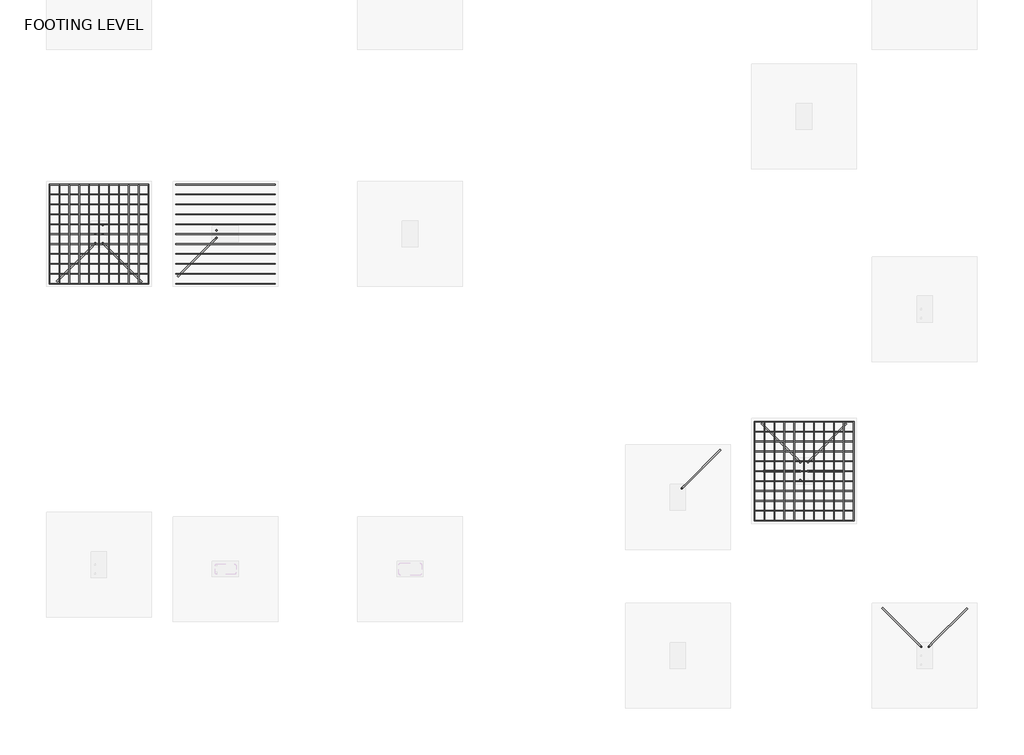
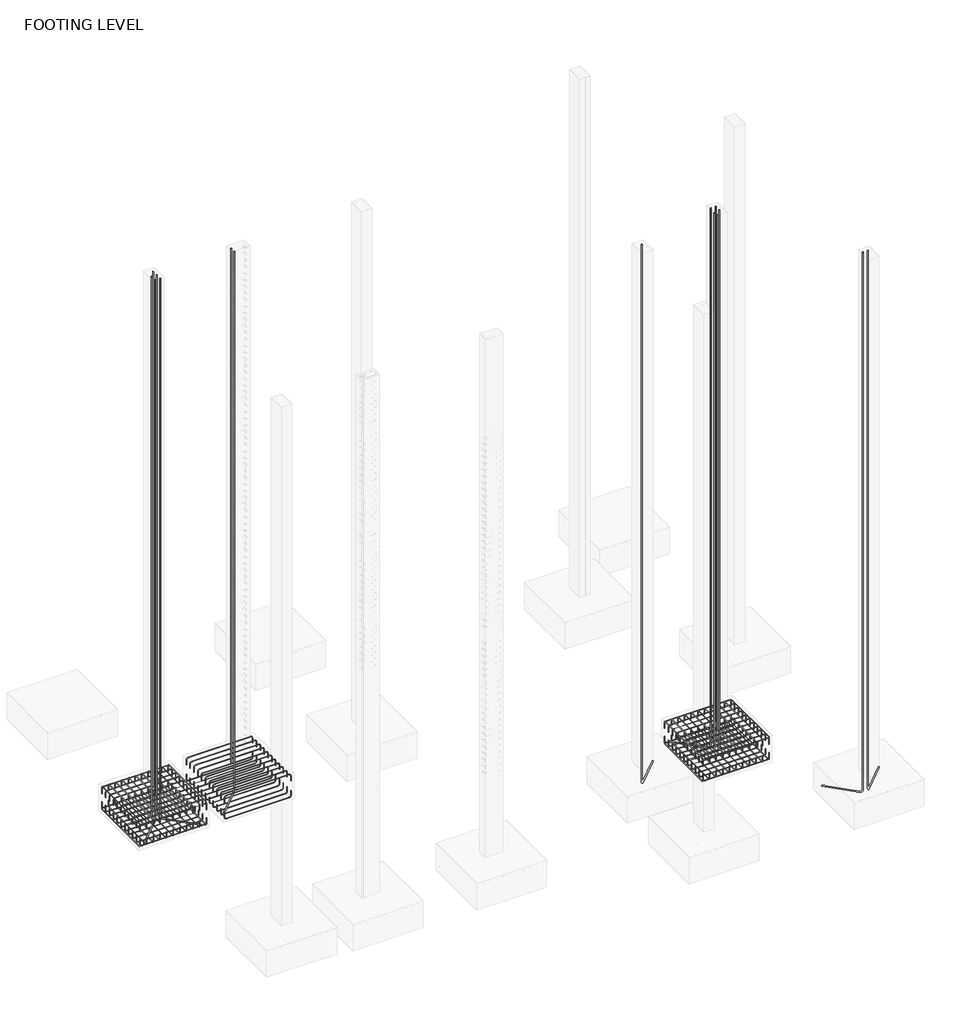
# One storey, part 7 of 10: 29 reinforcing bars.
"""IFC4 building model written with IfcOpenShell, lengths in millimetres."""

from ifc_helpers import new_model, si_unit, point, frame, origin, place, context, project, spatial, polyline, circle_curve, trimmed, segment, composite_curve, source, transform, mapped, element, save
from ifc_brep_helpers import swept_disk

model = new_model("IFC4")

# Units and contexts
model_context = context("Model", 3, world=origin())
ifc_project = project(units=[si_unit("LENGTHUNIT", "METRE", prefix="MILLI")], contexts=[model_context])

# Site, building, storey
site = spatial("IfcSite", under=ifc_project)
building = spatial("IfcBuilding", under=site)
storey = spatial("IfcBuildingStorey", under=building, Name="FOOTING LEVEL", Elevation=-1371.6)

# Reinforcing bars
placement = place(None, origin())
reinforcing_bar_shape = source(origin(), model_context, "Body", "SolidModel", [
    swept_disk(composite_curve([segment(polyline([(-13596.5793223, 10511.7953802, -1562.1), (-13596.5793223, 10511.7953802, -1447.8)]), True, "CONTINUOUS"), segment(trimmed(circle_curve(frame((-13563.2418223, 10511.7953802, -1447.8), z_axis=(0.0, 1.0, 0.0), x_axis=(-33.337499999999636, 0.0, 0.0)), 33.3375), [point((-13596.5793223, 10511.7953802, -1447.8))], [point((-13563.2418223, 10511.7953802, -1414.4625))], True, "CARTESIAN"), True, "CONTINUOUS"), segment(polyline([(-13563.2418223, 10511.7953802, -1414.4625), (-12191.6418223, 10511.7953802, -1414.4625)]), True, "CONTINUOUS"), segment(trimmed(circle_curve(frame((-12191.6418223, 10511.7953802, -1447.8), z_axis=(0.0, 1.0, 0.0), x_axis=(0.0, 0.0, 33.337499999999864)), 33.3375), [point((-12191.6418223, 10511.7953802, -1414.4625))], [point((-12158.3043223, 10511.7953802, -1447.8))], True, "CARTESIAN"), True, "CONTINUOUS"), segment(polyline([(-12158.3043223, 10511.7953802, -1447.8), (-12158.3043223, 10511.7953802, -1562.1)]), True, "CONTINUOUS")], self_intersect=False), 4.7625),
])
element("IfcReinforcingBar", 1, at=placement, inside=storey, context=model_context, shape_type="MappedRepresentation", body=[
    mapped(reinforcing_bar_shape, transform((0.0, 0.0, 0.0), x_axis=(1.0, 0.0, 0.0), y_axis=(0.0, 1.0, 0.0), z_axis=(0.0, 0.0, 1.0))),
    mapped(reinforcing_bar_shape, transform((0.0, -143.8275, 0.0), x_axis=(1.0, 0.0, 0.0), y_axis=(0.0, 1.0, 0.0), z_axis=(0.0, 0.0, 1.0))),
    mapped(reinforcing_bar_shape, transform((0.0, -287.655, 0.0), x_axis=(1.0, 0.0, 0.0), y_axis=(0.0, 1.0, 0.0), z_axis=(0.0, 0.0, 1.0))),
    mapped(reinforcing_bar_shape, transform((0.0, -431.4825, 0.0), x_axis=(1.0, 0.0, 0.0), y_axis=(0.0, 1.0, 0.0), z_axis=(0.0, 0.0, 1.0))),
    mapped(reinforcing_bar_shape, transform((0.0, -575.31, 0.0), x_axis=(1.0, 0.0, 0.0), y_axis=(0.0, 1.0, 0.0), z_axis=(0.0, 0.0, 1.0))),
    mapped(reinforcing_bar_shape, transform((0.0, -719.1375, 0.0), x_axis=(1.0, 0.0, 0.0), y_axis=(0.0, 1.0, 0.0), z_axis=(0.0, 0.0, 1.0))),
    mapped(reinforcing_bar_shape, transform((0.0, -862.965, 0.0), x_axis=(1.0, 0.0, 0.0), y_axis=(0.0, 1.0, 0.0), z_axis=(0.0, 0.0, 1.0))),
    mapped(reinforcing_bar_shape, transform((0.0, -1006.7925, 0.0), x_axis=(1.0, 0.0, 0.0), y_axis=(0.0, 1.0, 0.0), z_axis=(0.0, 0.0, 1.0))),
    mapped(reinforcing_bar_shape, transform((0.0, -1150.62, 0.0), x_axis=(1.0, 0.0, 0.0), y_axis=(0.0, 1.0, 0.0), z_axis=(0.0, 0.0, 1.0))),
    mapped(reinforcing_bar_shape, transform((0.0, -1294.4475, 0.0), x_axis=(1.0, 0.0, 0.0), y_axis=(0.0, 1.0, 0.0), z_axis=(0.0, 0.0, 1.0))),
    mapped(reinforcing_bar_shape, transform((0.0, -1438.275, 0.0), x_axis=(1.0, 0.0, 0.0), y_axis=(0.0, 1.0, 0.0), z_axis=(0.0, 0.0, 1.0))),
])
reinforcing_bar_2_shape = source(origin(), model_context, "Body", "SolidModel", [
    swept_disk(composite_curve([segment(polyline([(-12158.3043223, 10511.7953802, -1790.7), (-12158.3043223, 10511.7953802, -1905.0)]), True, "CONTINUOUS"), segment(trimmed(circle_curve(frame((-12191.6418223, 10511.7953802, -1905.0), z_axis=(0.0, 1.0, 0.0), x_axis=(33.337499999999636, 0.0, 0.0)), 33.3375), [point((-12158.3043223, 10511.7953802, -1905.0))], [point((-12191.6418223, 10511.7953802, -1938.3375))], True, "CARTESIAN"), True, "CONTINUOUS"), segment(polyline([(-12191.6418223, 10511.7953802, -1938.3375), (-13563.2418223, 10511.7953802, -1938.3375)]), True, "CONTINUOUS"), segment(trimmed(circle_curve(frame((-13563.2418223, 10511.7953802, -1905.0), z_axis=(0.0, 1.0, 0.0), x_axis=(0.0, 0.0, -33.33750000000009)), 33.3375), [point((-13563.2418223, 10511.7953802, -1938.3375))], [point((-13596.5793223, 10511.7953802, -1905.0))], True, "CARTESIAN"), True, "CONTINUOUS"), segment(polyline([(-13596.5793223, 10511.7953802, -1905.0), (-13596.5793223, 10511.7953802, -1790.7)]), True, "CONTINUOUS")], self_intersect=False), 4.7625),
])
element("IfcReinforcingBar", 2, at=placement, inside=storey, context=model_context, shape_type="MappedRepresentation", body=[
    mapped(reinforcing_bar_2_shape, transform((0.0, 0.0, 0.0), x_axis=(1.0, 0.0, 0.0), y_axis=(0.0, 1.0, 0.0), z_axis=(0.0, 0.0, 1.0))),
    mapped(reinforcing_bar_2_shape, transform((0.0, -143.8275, 0.0), x_axis=(1.0, 0.0, 0.0), y_axis=(0.0, 1.0, 0.0), z_axis=(0.0, 0.0, 1.0))),
    mapped(reinforcing_bar_2_shape, transform((0.0, -287.655, 0.0), x_axis=(1.0, 0.0, 0.0), y_axis=(0.0, 1.0, 0.0), z_axis=(0.0, 0.0, 1.0))),
    mapped(reinforcing_bar_2_shape, transform((0.0, -431.4825, 0.0), x_axis=(1.0, 0.0, 0.0), y_axis=(0.0, 1.0, 0.0), z_axis=(0.0, 0.0, 1.0))),
    mapped(reinforcing_bar_2_shape, transform((0.0, -575.31, 0.0), x_axis=(1.0, 0.0, 0.0), y_axis=(0.0, 1.0, 0.0), z_axis=(0.0, 0.0, 1.0))),
    mapped(reinforcing_bar_2_shape, transform((0.0, -719.1375, 0.0), x_axis=(1.0, 0.0, 0.0), y_axis=(0.0, 1.0, 0.0), z_axis=(0.0, 0.0, 1.0))),
    mapped(reinforcing_bar_2_shape, transform((0.0, -862.965, 0.0), x_axis=(1.0, 0.0, 0.0), y_axis=(0.0, 1.0, 0.0), z_axis=(0.0, 0.0, 1.0))),
    mapped(reinforcing_bar_2_shape, transform((0.0, -1006.7925, 0.0), x_axis=(1.0, 0.0, 0.0), y_axis=(0.0, 1.0, 0.0), z_axis=(0.0, 0.0, 1.0))),
    mapped(reinforcing_bar_2_shape, transform((0.0, -1150.62, 0.0), x_axis=(1.0, 0.0, 0.0), y_axis=(0.0, 1.0, 0.0), z_axis=(0.0, 0.0, 1.0))),
    mapped(reinforcing_bar_2_shape, transform((0.0, -1294.4475, 0.0), x_axis=(1.0, 0.0, 0.0), y_axis=(0.0, 1.0, 0.0), z_axis=(0.0, 0.0, 1.0))),
    mapped(reinforcing_bar_2_shape, transform((0.0, -1438.275, 0.0), x_axis=(1.0, 0.0, 0.0), y_axis=(0.0, 1.0, 0.0), z_axis=(0.0, 0.0, 1.0))),
])
reinforcing_bar_3_shape = source(origin(), model_context, "Body", "SolidModel", [
    swept_disk(composite_curve([segment(polyline([(-13993.4543223, 10511.7953802, -1562.1), (-13993.4543223, 10511.7953802, -1447.8)]), True, "CONTINUOUS"), segment(trimmed(circle_curve(frame((-13993.4543223, 10478.4578802, -1447.8), z_axis=(1.0, 0.0, 0.0), x_axis=(0.0, 33.337499999999636, 0.0)), 33.3375), [point((-13993.4543223, 10511.7953802, -1447.8))], [point((-13993.4543223, 10478.4578802, -1414.4625))], True, "CARTESIAN"), True, "CONTINUOUS"), segment(polyline([(-13993.4543223, 10478.4578802, -1414.4625), (-13993.4543223, 9106.8578802, -1414.4625)]), True, "CONTINUOUS"), segment(trimmed(circle_curve(frame((-13993.4543223, 9106.8578802, -1447.8), z_axis=(1.0, 0.0, 0.0), x_axis=(0.0, 0.0, 33.337499999999864)), 33.3375), [point((-13993.4543223, 9106.8578802, -1414.4625))], [point((-13993.4543223, 9073.5203802, -1447.8))], True, "CARTESIAN"), True, "CONTINUOUS"), segment(polyline([(-13993.4543223, 9073.5203802, -1447.8), (-13993.4543223, 9073.5203802, -1562.1)]), True, "CONTINUOUS")], self_intersect=False), 4.7625),
])
element("IfcReinforcingBar", 3, at=placement, inside=storey, context=model_context, shape_type="MappedRepresentation", body=[
    mapped(reinforcing_bar_3_shape, transform((0.0, 0.0, 0.0), x_axis=(1.0, 0.0, 0.0), y_axis=(0.0, 1.0, 0.0), z_axis=(0.0, 0.0, 1.0))),
    mapped(reinforcing_bar_3_shape, transform((-143.8275, 0.0, 0.0), x_axis=(1.0, 0.0, 0.0), y_axis=(0.0, 1.0, 0.0), z_axis=(0.0, 0.0, 1.0))),
    mapped(reinforcing_bar_3_shape, transform((-287.655, 0.0, 0.0), x_axis=(1.0, 0.0, 0.0), y_axis=(0.0, 1.0, 0.0), z_axis=(0.0, 0.0, 1.0))),
    mapped(reinforcing_bar_3_shape, transform((-431.4825, 0.0, 0.0), x_axis=(1.0, 0.0, 0.0), y_axis=(0.0, 1.0, 0.0), z_axis=(0.0, 0.0, 1.0))),
    mapped(reinforcing_bar_3_shape, transform((-575.31, 0.0, 0.0), x_axis=(1.0, 0.0, 0.0), y_axis=(0.0, 1.0, 0.0), z_axis=(0.0, 0.0, 1.0))),
    mapped(reinforcing_bar_3_shape, transform((-719.1375, 0.0, 0.0), x_axis=(1.0, 0.0, 0.0), y_axis=(0.0, 1.0, 0.0), z_axis=(0.0, 0.0, 1.0))),
    mapped(reinforcing_bar_3_shape, transform((-862.965, 0.0, 0.0), x_axis=(1.0, 0.0, 0.0), y_axis=(0.0, 1.0, 0.0), z_axis=(0.0, 0.0, 1.0))),
    mapped(reinforcing_bar_3_shape, transform((-1006.7925, 0.0, 0.0), x_axis=(1.0, 0.0, 0.0), y_axis=(0.0, 1.0, 0.0), z_axis=(0.0, 0.0, 1.0))),
    mapped(reinforcing_bar_3_shape, transform((-1150.62, 0.0, 0.0), x_axis=(1.0, 0.0, 0.0), y_axis=(0.0, 1.0, 0.0), z_axis=(0.0, 0.0, 1.0))),
    mapped(reinforcing_bar_3_shape, transform((-1294.4475, 0.0, 0.0), x_axis=(1.0, 0.0, 0.0), y_axis=(0.0, 1.0, 0.0), z_axis=(0.0, 0.0, 1.0))),
    mapped(reinforcing_bar_3_shape, transform((-1438.275, 0.0, 0.0), x_axis=(1.0, 0.0, 0.0), y_axis=(0.0, 1.0, 0.0), z_axis=(0.0, 0.0, 1.0))),
])
reinforcing_bar_4_shape = source(origin(), model_context, "Body", "SolidModel", [
    swept_disk(composite_curve([segment(polyline([(-13993.4543223, 9073.5203802, -1790.7), (-13993.4543223, 9073.5203802, -1905.0)]), True, "CONTINUOUS"), segment(trimmed(circle_curve(frame((-13993.4543223, 9106.8578802, -1905.0), z_axis=(1.0, 0.0, 0.0), x_axis=(0.0, -33.337499999999636, 0.0)), 33.3375), [point((-13993.4543223, 9073.5203802, -1905.0))], [point((-13993.4543223, 9106.8578802, -1938.3375))], True, "CARTESIAN"), True, "CONTINUOUS"), segment(polyline([(-13993.4543223, 9106.8578802, -1938.3375), (-13993.4543223, 10478.4578802, -1938.3375)]), True, "CONTINUOUS"), segment(trimmed(circle_curve(frame((-13993.4543223, 10478.4578802, -1905.0), z_axis=(1.0, 0.0, 0.0), x_axis=(0.0, 0.0, -33.33750000000009)), 33.3375), [point((-13993.4543223, 10478.4578802, -1938.3375))], [point((-13993.4543223, 10511.7953802, -1905.0))], True, "CARTESIAN"), True, "CONTINUOUS"), segment(polyline([(-13993.4543223, 10511.7953802, -1905.0), (-13993.4543223, 10511.7953802, -1790.7)]), True, "CONTINUOUS")], self_intersect=False), 4.7625),
])
element("IfcReinforcingBar", 4, at=placement, inside=storey, context=model_context, shape_type="MappedRepresentation", body=[
    mapped(reinforcing_bar_4_shape, transform((0.0, 0.0, 0.0), x_axis=(1.0, 0.0, 0.0), y_axis=(0.0, 1.0, 0.0), z_axis=(0.0, 0.0, 1.0))),
    mapped(reinforcing_bar_4_shape, transform((-143.8275, 0.0, 0.0), x_axis=(1.0, 0.0, 0.0), y_axis=(0.0, 1.0, 0.0), z_axis=(0.0, 0.0, 1.0))),
    mapped(reinforcing_bar_4_shape, transform((-287.655, 0.0, 0.0), x_axis=(1.0, 0.0, 0.0), y_axis=(0.0, 1.0, 0.0), z_axis=(0.0, 0.0, 1.0))),
    mapped(reinforcing_bar_4_shape, transform((-431.4825, 0.0, 0.0), x_axis=(1.0, 0.0, 0.0), y_axis=(0.0, 1.0, 0.0), z_axis=(0.0, 0.0, 1.0))),
    mapped(reinforcing_bar_4_shape, transform((-575.31, 0.0, 0.0), x_axis=(1.0, 0.0, 0.0), y_axis=(0.0, 1.0, 0.0), z_axis=(0.0, 0.0, 1.0))),
    mapped(reinforcing_bar_4_shape, transform((-719.1375, 0.0, 0.0), x_axis=(1.0, 0.0, 0.0), y_axis=(0.0, 1.0, 0.0), z_axis=(0.0, 0.0, 1.0))),
    mapped(reinforcing_bar_4_shape, transform((-862.965, 0.0, 0.0), x_axis=(1.0, 0.0, 0.0), y_axis=(0.0, 1.0, 0.0), z_axis=(0.0, 0.0, 1.0))),
    mapped(reinforcing_bar_4_shape, transform((-1006.7925, 0.0, 0.0), x_axis=(1.0, 0.0, 0.0), y_axis=(0.0, 1.0, 0.0), z_axis=(0.0, 0.0, 1.0))),
    mapped(reinforcing_bar_4_shape, transform((-1150.62, 0.0, 0.0), x_axis=(1.0, 0.0, 0.0), y_axis=(0.0, 1.0, 0.0), z_axis=(0.0, 0.0, 1.0))),
    mapped(reinforcing_bar_4_shape, transform((-1294.4475, 0.0, 0.0), x_axis=(1.0, 0.0, 0.0), y_axis=(0.0, 1.0, 0.0), z_axis=(0.0, 0.0, 1.0))),
    mapped(reinforcing_bar_4_shape, transform((-1438.275, 0.0, 0.0), x_axis=(1.0, 0.0, 0.0), y_axis=(0.0, 1.0, 0.0), z_axis=(0.0, 0.0, 1.0))),
])
reinforcing_bar_5_shape = source(origin(), model_context, "Body", "SolidModel", [
    swept_disk(composite_curve([segment(polyline([(-15431.7293223, 9073.5203802, -1770.864029), (-15431.7293223, 9073.5203802, -1885.164029)]), True, "CONTINUOUS"), segment(trimmed(circle_curve(frame((-15398.3918223, 9073.5203802, -1885.164029), z_axis=(0.0, -1.0, 0.0), x_axis=(-33.337499999999636, 0.0, 0.0)), 33.3375), [point((-15431.7293223, 9073.5203802, -1885.164029))], [point((-15398.3918223, 9073.5203802, -1918.501529))], True, "CARTESIAN"), True, "CONTINUOUS"), segment(polyline([(-15398.3918223, 9073.5203802, -1918.501529), (-14026.7918223, 9073.5203802, -1918.501529)]), True, "CONTINUOUS"), segment(trimmed(circle_curve(frame((-14026.7918223, 9073.5203802, -1885.164029), z_axis=(0.0, -1.0, 0.0), x_axis=(0.0, 0.0, -33.337499999999864)), 33.3375), [point((-14026.7918223, 9073.5203802, -1918.501529))], [point((-13993.4543223, 9073.5203802, -1885.164029))], True, "CARTESIAN"), True, "CONTINUOUS"), segment(polyline([(-13993.4543223, 9073.5203802, -1885.164029), (-13993.4543223, 9073.5203802, -1770.864029)]), True, "CONTINUOUS")], self_intersect=False), 4.7625),
])
element("IfcReinforcingBar", 5, at=placement, inside=storey, context=model_context, shape_type="MappedRepresentation", body=[
    mapped(reinforcing_bar_5_shape, transform((0.0, 0.0, 0.0), x_axis=(1.0, 0.0, 0.0), y_axis=(0.0, 1.0, 0.0), z_axis=(0.0, 0.0, 1.0))),
    mapped(reinforcing_bar_5_shape, transform((0.0, 143.8275, 0.0), x_axis=(1.0, 0.0, 0.0), y_axis=(0.0, 1.0, 0.0), z_axis=(0.0, 0.0, 1.0))),
    mapped(reinforcing_bar_5_shape, transform((0.0, 287.655, 0.0), x_axis=(1.0, 0.0, 0.0), y_axis=(0.0, 1.0, 0.0), z_axis=(0.0, 0.0, 1.0))),
    mapped(reinforcing_bar_5_shape, transform((0.0, 431.4825, 0.0), x_axis=(1.0, 0.0, 0.0), y_axis=(0.0, 1.0, 0.0), z_axis=(0.0, 0.0, 1.0))),
    mapped(reinforcing_bar_5_shape, transform((0.0, 575.31, 0.0), x_axis=(1.0, 0.0, 0.0), y_axis=(0.0, 1.0, 0.0), z_axis=(0.0, 0.0, 1.0))),
    mapped(reinforcing_bar_5_shape, transform((0.0, 719.1375, 0.0), x_axis=(1.0, 0.0, 0.0), y_axis=(0.0, 1.0, 0.0), z_axis=(0.0, 0.0, 1.0))),
    mapped(reinforcing_bar_5_shape, transform((0.0, 862.965, 0.0), x_axis=(1.0, 0.0, 0.0), y_axis=(0.0, 1.0, 0.0), z_axis=(0.0, 0.0, 1.0))),
    mapped(reinforcing_bar_5_shape, transform((0.0, 1006.7925, 0.0), x_axis=(1.0, 0.0, 0.0), y_axis=(0.0, 1.0, 0.0), z_axis=(0.0, 0.0, 1.0))),
    mapped(reinforcing_bar_5_shape, transform((0.0, 1150.62, 0.0), x_axis=(1.0, 0.0, 0.0), y_axis=(0.0, 1.0, 0.0), z_axis=(0.0, 0.0, 1.0))),
    mapped(reinforcing_bar_5_shape, transform((0.0, 1294.4475, 0.0), x_axis=(1.0, 0.0, 0.0), y_axis=(0.0, 1.0, 0.0), z_axis=(0.0, 0.0, 1.0))),
    mapped(reinforcing_bar_5_shape, transform((0.0, 1438.275, 0.0), x_axis=(1.0, 0.0, 0.0), y_axis=(0.0, 1.0, 0.0), z_axis=(0.0, 0.0, 1.0))),
])
reinforcing_bar_6_shape = source(origin(), model_context, "Body", "SolidModel", [
    swept_disk(composite_curve([segment(polyline([(-15431.7293223, 10511.7953802, -1586.5406765), (-15431.7293223, 10511.7953802, -1472.2406765)]), True, "CONTINUOUS"), segment(trimmed(circle_curve(frame((-15398.3918223, 10511.7953802, -1472.2406765), z_axis=(0.0, 1.0, 0.0), x_axis=(-33.337499999999636, 0.0, 0.0)), 33.3375), [point((-15431.7293223, 10511.7953802, -1472.2406765))], [point((-15398.3918223, 10511.7953802, -1438.9031765))], True, "CARTESIAN"), True, "CONTINUOUS"), segment(polyline([(-15398.3918223, 10511.7953802, -1438.9031765), (-14026.7918223, 10511.7953802, -1438.9031765)]), True, "CONTINUOUS"), segment(trimmed(circle_curve(frame((-14026.7918223, 10511.7953802, -1472.2406765), z_axis=(0.0, 1.0, 0.0), x_axis=(0.0, 0.0, 33.33750000000009)), 33.3375), [point((-14026.7918223, 10511.7953802, -1438.9031765))], [point((-13993.4543223, 10511.7953802, -1472.2406765))], True, "CARTESIAN"), True, "CONTINUOUS"), segment(polyline([(-13993.4543223, 10511.7953802, -1472.2406765), (-13993.4543223, 10511.7953802, -1586.5406765)]), True, "CONTINUOUS")], self_intersect=False), 4.7625),
])
element("IfcReinforcingBar", 6, at=placement, inside=storey, context=model_context, shape_type="MappedRepresentation", body=[
    mapped(reinforcing_bar_6_shape, transform((0.0, 0.0, 0.0), x_axis=(1.0, 0.0, 0.0), y_axis=(0.0, 1.0, 0.0), z_axis=(0.0, 0.0, 1.0))),
    mapped(reinforcing_bar_6_shape, transform((0.0, -143.8275, 0.0), x_axis=(1.0, 0.0, 0.0), y_axis=(0.0, 1.0, 0.0), z_axis=(0.0, 0.0, 1.0))),
    mapped(reinforcing_bar_6_shape, transform((0.0, -287.655, 0.0), x_axis=(1.0, 0.0, 0.0), y_axis=(0.0, 1.0, 0.0), z_axis=(0.0, 0.0, 1.0))),
    mapped(reinforcing_bar_6_shape, transform((0.0, -431.4825, 0.0), x_axis=(1.0, 0.0, 0.0), y_axis=(0.0, 1.0, 0.0), z_axis=(0.0, 0.0, 1.0))),
    mapped(reinforcing_bar_6_shape, transform((0.0, -575.31, 0.0), x_axis=(1.0, 0.0, 0.0), y_axis=(0.0, 1.0, 0.0), z_axis=(0.0, 0.0, 1.0))),
    mapped(reinforcing_bar_6_shape, transform((0.0, -719.1375, 0.0), x_axis=(1.0, 0.0, 0.0), y_axis=(0.0, 1.0, 0.0), z_axis=(0.0, 0.0, 1.0))),
    mapped(reinforcing_bar_6_shape, transform((0.0, -862.965, 0.0), x_axis=(1.0, 0.0, 0.0), y_axis=(0.0, 1.0, 0.0), z_axis=(0.0, 0.0, 1.0))),
    mapped(reinforcing_bar_6_shape, transform((0.0, -1006.7925, 0.0), x_axis=(1.0, 0.0, 0.0), y_axis=(0.0, 1.0, 0.0), z_axis=(0.0, 0.0, 1.0))),
    mapped(reinforcing_bar_6_shape, transform((0.0, -1150.62, 0.0), x_axis=(1.0, 0.0, 0.0), y_axis=(0.0, 1.0, 0.0), z_axis=(0.0, 0.0, 1.0))),
    mapped(reinforcing_bar_6_shape, transform((0.0, -1294.4475, 0.0), x_axis=(1.0, 0.0, 0.0), y_axis=(0.0, 1.0, 0.0), z_axis=(0.0, 0.0, 1.0))),
    mapped(reinforcing_bar_6_shape, transform((0.0, -1438.275, 0.0), x_axis=(1.0, 0.0, 0.0), y_axis=(0.0, 1.0, 0.0), z_axis=(0.0, 0.0, 1.0))),
])
reinforcing_bar_7_shape = source(origin(), model_context, "Body", "SolidModel", [
    swept_disk(composite_curve([segment(polyline([(-5201.8793223, 5631.8203802, -1562.1), (-5201.8793223, 5631.8203802, -1447.8)]), True, "CONTINUOUS"), segment(trimmed(circle_curve(frame((-5201.8793223, 5665.1578802, -1447.8), z_axis=(-1.0, 0.0, 0.0), x_axis=(0.0, -33.337500000000546, 0.0)), 33.3375), [point((-5201.8793223, 5631.8203802, -1447.8))], [point((-5201.8793223, 5665.1578802, -1414.4625))], True, "CARTESIAN"), True, "CONTINUOUS"), segment(polyline([(-5201.8793223, 5665.1578802, -1414.4625), (-5201.8793223, 7036.7578802, -1414.4625)]), True, "CONTINUOUS"), segment(trimmed(circle_curve(frame((-5201.8793223, 7036.7578802, -1447.8), z_axis=(-1.0, 0.0, 0.0), x_axis=(0.0, 0.0, 33.337499999999864)), 33.3375), [point((-5201.8793223, 7036.7578802, -1414.4625))], [point((-5201.8793223, 7070.0953802, -1447.8))], True, "CARTESIAN"), True, "CONTINUOUS"), segment(polyline([(-5201.8793223, 7070.0953802, -1447.8), (-5201.8793223, 7070.0953802, -1562.1)]), True, "CONTINUOUS")], self_intersect=False), 4.7625),
])
element("IfcReinforcingBar", 7, at=placement, inside=storey, context=model_context, shape_type="MappedRepresentation", body=[
    mapped(reinforcing_bar_7_shape, transform((0.0, 0.0, 0.0), x_axis=(1.0, 0.0, 0.0), y_axis=(0.0, 1.0, 0.0), z_axis=(0.0, 0.0, 1.0))),
    mapped(reinforcing_bar_7_shape, transform((143.8275, 0.0, 0.0), x_axis=(1.0, 0.0, 0.0), y_axis=(0.0, 1.0, 0.0), z_axis=(0.0, 0.0, 1.0))),
    mapped(reinforcing_bar_7_shape, transform((287.655, 0.0, 0.0), x_axis=(1.0, 0.0, 0.0), y_axis=(0.0, 1.0, 0.0), z_axis=(0.0, 0.0, 1.0))),
    mapped(reinforcing_bar_7_shape, transform((431.4825, 0.0, 0.0), x_axis=(1.0, 0.0, 0.0), y_axis=(0.0, 1.0, 0.0), z_axis=(0.0, 0.0, 1.0))),
    mapped(reinforcing_bar_7_shape, transform((575.31, 0.0, 0.0), x_axis=(1.0, 0.0, 0.0), y_axis=(0.0, 1.0, 0.0), z_axis=(0.0, 0.0, 1.0))),
    mapped(reinforcing_bar_7_shape, transform((719.1375, 0.0, 0.0), x_axis=(1.0, 0.0, 0.0), y_axis=(0.0, 1.0, 0.0), z_axis=(0.0, 0.0, 1.0))),
    mapped(reinforcing_bar_7_shape, transform((862.965, 0.0, 0.0), x_axis=(1.0, 0.0, 0.0), y_axis=(0.0, 1.0, 0.0), z_axis=(0.0, 0.0, 1.0))),
    mapped(reinforcing_bar_7_shape, transform((1006.7925, 0.0, 0.0), x_axis=(1.0, 0.0, 0.0), y_axis=(0.0, 1.0, 0.0), z_axis=(0.0, 0.0, 1.0))),
    mapped(reinforcing_bar_7_shape, transform((1150.62, 0.0, 0.0), x_axis=(1.0, 0.0, 0.0), y_axis=(0.0, 1.0, 0.0), z_axis=(0.0, 0.0, 1.0))),
    mapped(reinforcing_bar_7_shape, transform((1294.4475, 0.0, 0.0), x_axis=(1.0, 0.0, 0.0), y_axis=(0.0, 1.0, 0.0), z_axis=(0.0, 0.0, 1.0))),
    mapped(reinforcing_bar_7_shape, transform((1438.275, 0.0, 0.0), x_axis=(1.0, 0.0, 0.0), y_axis=(0.0, 1.0, 0.0), z_axis=(0.0, 0.0, 1.0))),
])
reinforcing_bar_8_shape = source(origin(), model_context, "Body", "SolidModel", [
    swept_disk(composite_curve([segment(polyline([(-5201.8793223, 7070.0953802, -1790.7), (-5201.8793223, 7070.0953802, -1905.0)]), True, "CONTINUOUS"), segment(trimmed(circle_curve(frame((-5201.8793223, 7036.7578802, -1905.0), z_axis=(-1.0, 0.0, 0.0), x_axis=(0.0, 33.337500000000546, 0.0)), 33.3375), [point((-5201.8793223, 7070.0953802, -1905.0))], [point((-5201.8793223, 7036.7578802, -1938.3375))], True, "CARTESIAN"), True, "CONTINUOUS"), segment(polyline([(-5201.8793223, 7036.7578802, -1938.3375), (-5201.8793223, 5665.1578802, -1938.3375)]), True, "CONTINUOUS"), segment(trimmed(circle_curve(frame((-5201.8793223, 5665.1578802, -1905.0), z_axis=(-1.0, 0.0, 0.0), x_axis=(0.0, 0.0, -33.33750000000009)), 33.3375), [point((-5201.8793223, 5665.1578802, -1938.3375))], [point((-5201.8793223, 5631.8203802, -1905.0))], True, "CARTESIAN"), True, "CONTINUOUS"), segment(polyline([(-5201.8793223, 5631.8203802, -1905.0), (-5201.8793223, 5631.8203802, -1790.7)]), True, "CONTINUOUS")], self_intersect=False), 4.7625),
])
element("IfcReinforcingBar", 8, at=placement, inside=storey, context=model_context, shape_type="MappedRepresentation", body=[
    mapped(reinforcing_bar_8_shape, transform((0.0, 0.0, 0.0), x_axis=(1.0, 0.0, 0.0), y_axis=(0.0, 1.0, 0.0), z_axis=(0.0, 0.0, 1.0))),
    mapped(reinforcing_bar_8_shape, transform((143.8275, 0.0, 0.0), x_axis=(1.0, 0.0, 0.0), y_axis=(0.0, 1.0, 0.0), z_axis=(0.0, 0.0, 1.0))),
    mapped(reinforcing_bar_8_shape, transform((287.655, 0.0, 0.0), x_axis=(1.0, 0.0, 0.0), y_axis=(0.0, 1.0, 0.0), z_axis=(0.0, 0.0, 1.0))),
    mapped(reinforcing_bar_8_shape, transform((431.4825, 0.0, 0.0), x_axis=(1.0, 0.0, 0.0), y_axis=(0.0, 1.0, 0.0), z_axis=(0.0, 0.0, 1.0))),
    mapped(reinforcing_bar_8_shape, transform((575.31, 0.0, 0.0), x_axis=(1.0, 0.0, 0.0), y_axis=(0.0, 1.0, 0.0), z_axis=(0.0, 0.0, 1.0))),
    mapped(reinforcing_bar_8_shape, transform((719.1375, 0.0, 0.0), x_axis=(1.0, 0.0, 0.0), y_axis=(0.0, 1.0, 0.0), z_axis=(0.0, 0.0, 1.0))),
    mapped(reinforcing_bar_8_shape, transform((862.965, 0.0, 0.0), x_axis=(1.0, 0.0, 0.0), y_axis=(0.0, 1.0, 0.0), z_axis=(0.0, 0.0, 1.0))),
    mapped(reinforcing_bar_8_shape, transform((1006.7925, 0.0, 0.0), x_axis=(1.0, 0.0, 0.0), y_axis=(0.0, 1.0, 0.0), z_axis=(0.0, 0.0, 1.0))),
    mapped(reinforcing_bar_8_shape, transform((1150.62, 0.0, 0.0), x_axis=(1.0, 0.0, 0.0), y_axis=(0.0, 1.0, 0.0), z_axis=(0.0, 0.0, 1.0))),
    mapped(reinforcing_bar_8_shape, transform((1294.4475, 0.0, 0.0), x_axis=(1.0, 0.0, 0.0), y_axis=(0.0, 1.0, 0.0), z_axis=(0.0, 0.0, 1.0))),
    mapped(reinforcing_bar_8_shape, transform((1438.275, 0.0, 0.0), x_axis=(1.0, 0.0, 0.0), y_axis=(0.0, 1.0, 0.0), z_axis=(0.0, 0.0, 1.0))),
])
reinforcing_bar_9_shape = source(origin(), model_context, "Body", "SolidModel", [
    swept_disk(composite_curve([segment(polyline([(-3763.6043223, 7070.0953802, -1770.864029), (-3763.6043223, 7070.0953802, -1885.164029)]), True, "CONTINUOUS"), segment(trimmed(circle_curve(frame((-3796.9418223, 7070.0953802, -1885.164029), z_axis=(0.0, 1.0, 0.0), x_axis=(33.337499999999636, 0.0, 0.0)), 33.3375), [point((-3763.6043223, 7070.0953802, -1885.164029))], [point((-3796.9418223, 7070.0953802, -1918.501529))], True, "CARTESIAN"), True, "CONTINUOUS"), segment(polyline([(-3796.9418223, 7070.0953802, -1918.501529), (-5168.5418223, 7070.0953802, -1918.501529)]), True, "CONTINUOUS"), segment(trimmed(circle_curve(frame((-5168.5418223, 7070.0953802, -1885.164029), z_axis=(0.0, 1.0, 0.0), x_axis=(0.0, 0.0, -33.337499999999864)), 33.3375), [point((-5168.5418223, 7070.0953802, -1918.501529))], [point((-5201.8793223, 7070.0953802, -1885.164029))], True, "CARTESIAN"), True, "CONTINUOUS"), segment(polyline([(-5201.8793223, 7070.0953802, -1885.164029), (-5201.8793223, 7070.0953802, -1770.864029)]), True, "CONTINUOUS")], self_intersect=False), 4.7625),
])
element("IfcReinforcingBar", 9, at=placement, inside=storey, context=model_context, shape_type="MappedRepresentation", body=[
    mapped(reinforcing_bar_9_shape, transform((0.0, 0.0, 0.0), x_axis=(1.0, 0.0, 0.0), y_axis=(0.0, 1.0, 0.0), z_axis=(0.0, 0.0, 1.0))),
    mapped(reinforcing_bar_9_shape, transform((0.0, -143.8275, 0.0), x_axis=(1.0, 0.0, 0.0), y_axis=(0.0, 1.0, 0.0), z_axis=(0.0, 0.0, 1.0))),
    mapped(reinforcing_bar_9_shape, transform((0.0, -287.655, 0.0), x_axis=(1.0, 0.0, 0.0), y_axis=(0.0, 1.0, 0.0), z_axis=(0.0, 0.0, 1.0))),
    mapped(reinforcing_bar_9_shape, transform((0.0, -431.4825, 0.0), x_axis=(1.0, 0.0, 0.0), y_axis=(0.0, 1.0, 0.0), z_axis=(0.0, 0.0, 1.0))),
    mapped(reinforcing_bar_9_shape, transform((0.0, -575.31, 0.0), x_axis=(1.0, 0.0, 0.0), y_axis=(0.0, 1.0, 0.0), z_axis=(0.0, 0.0, 1.0))),
    mapped(reinforcing_bar_9_shape, transform((0.0, -719.1375, 0.0), x_axis=(1.0, 0.0, 0.0), y_axis=(0.0, 1.0, 0.0), z_axis=(0.0, 0.0, 1.0))),
    mapped(reinforcing_bar_9_shape, transform((0.0, -862.965, 0.0), x_axis=(1.0, 0.0, 0.0), y_axis=(0.0, 1.0, 0.0), z_axis=(0.0, 0.0, 1.0))),
    mapped(reinforcing_bar_9_shape, transform((0.0, -1006.7925, 0.0), x_axis=(1.0, 0.0, 0.0), y_axis=(0.0, 1.0, 0.0), z_axis=(0.0, 0.0, 1.0))),
    mapped(reinforcing_bar_9_shape, transform((0.0, -1150.62, 0.0), x_axis=(1.0, 0.0, 0.0), y_axis=(0.0, 1.0, 0.0), z_axis=(0.0, 0.0, 1.0))),
    mapped(reinforcing_bar_9_shape, transform((0.0, -1294.4475, 0.0), x_axis=(1.0, 0.0, 0.0), y_axis=(0.0, 1.0, 0.0), z_axis=(0.0, 0.0, 1.0))),
    mapped(reinforcing_bar_9_shape, transform((0.0, -1438.275, 0.0), x_axis=(1.0, 0.0, 0.0), y_axis=(0.0, 1.0, 0.0), z_axis=(0.0, 0.0, 1.0))),
])
element("IfcReinforcingBar", 10, at=placement, inside=storey, context=model_context, shape_type="SolidModel", body=[
    swept_disk(composite_curve([segment(polyline([(-14658.2316302, 9923.2180723, -1333.5), (-14658.2316302, 9923.2180723, 10477.5)]), True, "CONTINUOUS")], self_intersect=False), 9.525),
])
element("IfcReinforcingBar", 11, at=placement, inside=storey, context=model_context, shape_type="SolidModel", body=[
    swept_disk(composite_curve([segment(polyline([(-14766.9520144, 9662.0976881, -1333.5), (-14766.9520144, 9662.0976881, 10477.5)]), True, "CONTINUOUS")], self_intersect=False), 9.525),
])
element("IfcReinforcingBar", 12, at=placement, inside=storey, context=model_context, shape_type="SolidModel", body=[
    swept_disk(composite_curve([segment(polyline([(-14658.2316302, 9662.0976881, -1333.5), (-14658.2316302, 9662.0976881, 10477.5)]), True, "CONTINUOUS")], self_intersect=False), 9.525),
])
element("IfcReinforcingBar", 13, at=placement, inside=storey, context=model_context, shape_type="SolidModel", body=[
    swept_disk(composite_curve([segment(polyline([(-15325.6711349, 9103.3785676, -1910.4342608), (-14814.0983591, 9614.9513434, -1910.4342608)]), True, "CONTINUOUS"), segment(trimmed(circle_curve(frame((-14814.0983591, 9614.9513434, -1843.7592608), z_axis=(0.707106781186576, -0.7071067811865192, 0.0), x_axis=(0.0, 0.0, -66.67499999999995)), 66.675), [point((-14814.0983591, 9614.9513434, -1910.4342608))], [point((-14766.9520144, 9662.0976881, -1843.7592608))], True, "CARTESIAN"), True, "CONTINUOUS"), segment(polyline([(-14766.9520144, 9662.0976881, -1843.7592608), (-14766.9520144, 9662.0976881, 10477.5)]), True, "CONTINUOUS")], self_intersect=False), 9.525),
])
element("IfcReinforcingBar", 14, at=placement, inside=storey, context=model_context, shape_type="SolidModel", body=[
    swept_disk(composite_curve([segment(polyline([(-14094.0528099, 9097.9188678, -1910.4342608), (-14611.0852856, 9614.9513434, -1910.4342608)]), True, "CONTINUOUS"), segment(trimmed(circle_curve(frame((-14611.0852856, 9614.9513434, -1843.7592608), z_axis=(0.7071067811865689, 0.7071067811865261, 0.0), x_axis=(0.0, 0.0, -66.67499999999995)), 66.675), [point((-14611.0852856, 9614.9513434, -1910.4342608))], [point((-14658.2316302, 9662.0976881, -1843.7592608))], True, "CARTESIAN"), True, "CONTINUOUS"), segment(polyline([(-14658.2316302, 9662.0976881, -1843.7592608), (-14658.2316302, 9662.0976881, 10477.5)]), True, "CONTINUOUS")], self_intersect=False), 9.525),
])
element("IfcReinforcingBar", 15, at=placement, inside=storey, context=model_context, shape_type="SolidModel", body=[
    swept_disk(composite_curve([segment(polyline([(-15305.1818909, 9792.6578802, -1910.4342608), (-14833.6270144, 9792.6578802, -1910.4342608)]), True, "CONTINUOUS"), segment(trimmed(circle_curve(frame((-14833.6270144, 9792.6578802, -1843.7592608), z_axis=(0.0, -1.0, 0.0), x_axis=(0.0, 0.0, -66.67499999999995)), 66.675), [point((-14833.6270144, 9792.6578802, -1910.4342608))], [point((-14766.9520144, 9792.6578802, -1843.7592608))], True, "CARTESIAN"), True, "CONTINUOUS"), segment(polyline([(-14766.9520144, 9792.6578802, -1843.7592608), (-14766.9520144, 9792.6578802, 10477.5)]), True, "CONTINUOUS")], self_intersect=False), 9.525),
])
element("IfcReinforcingBar", 16, at=placement, inside=storey, context=model_context, shape_type="SolidModel", body=[
    swept_disk(composite_curve([segment(polyline([(-14120.0017538, 9792.6578802, -1910.4342608), (-14591.5566302, 9792.6578802, -1910.4342608)]), True, "CONTINUOUS"), segment(trimmed(circle_curve(frame((-14591.5566302, 9792.6578802, -1843.7592608), z_axis=(0.0, 1.0, 0.0), x_axis=(0.0, 0.0, -66.67499999999995)), 66.675), [point((-14591.5566302, 9792.6578802, -1910.4342608))], [point((-14658.2316302, 9792.6578802, -1843.7592608))], True, "CARTESIAN"), True, "CONTINUOUS"), segment(polyline([(-14658.2316302, 9792.6578802, -1843.7592608), (-14658.2316302, 9792.6578802, 10477.5)]), True, "CONTINUOUS")], self_intersect=False), 9.525),
])
element("IfcReinforcingBar", 17, at=placement, inside=storey, context=model_context, shape_type="SolidModel", body=[
    swept_disk(composite_curve([segment(polyline([(-2117.0625098, 4360.5371927, -1910.4342608), (-2628.6352856, 3848.9644169, -1910.4342608)]), True, "CONTINUOUS"), segment(trimmed(circle_curve(frame((-2628.6352856, 3848.9644169, -1843.7592608), z_axis=(-0.7071067811865738, 0.7071067811865214, 0.0), x_axis=(0.0, 0.0, -66.67499999999995)), 66.675), [point((-2628.6352856, 3848.9644169, -1910.4342608))], [point((-2675.7816302, 3801.8180723, -1843.7592608))], True, "CARTESIAN"), True, "CONTINUOUS"), segment(polyline([(-2675.7816302, 3801.8180723, -1843.7592608), (-2675.7816302, 3801.8180723, 10477.5)]), True, "CONTINUOUS")], self_intersect=False), 9.525),
])
element("IfcReinforcingBar", 18, at=placement, inside=storey, context=model_context, shape_type="SolidModel", body=[
    swept_disk(composite_curve([segment(polyline([(-3348.6808347, 4365.9968926, -1910.4342608), (-2831.6483591, 3848.9644169, -1910.4342608)]), True, "CONTINUOUS"), segment(trimmed(circle_curve(frame((-2831.6483591, 3848.9644169, -1843.7592608), z_axis=(-0.7071067811865711, -0.7071067811865239, 0.0), x_axis=(0.0, 0.0, -66.67499999999995)), 66.675), [point((-2831.6483591, 3848.9644169, -1910.4342608))], [point((-2784.5020144, 3801.8180723, -1843.7592608))], True, "CARTESIAN"), True, "CONTINUOUS"), segment(polyline([(-2784.5020144, 3801.8180723, -1843.7592608), (-2784.5020144, 3801.8180723, 10477.5)]), True, "CONTINUOUS")], self_intersect=False), 9.525),
])
element("IfcReinforcingBar", 19, at=placement, inside=storey, context=model_context, shape_type="SolidModel", body=[
    swept_disk(composite_curve([segment(polyline([(-5698.4625098, 6659.2371927, -1910.4342608), (-6210.0352856, 6147.6644169, -1910.4342608)]), True, "CONTINUOUS"), segment(trimmed(circle_curve(frame((-6210.0352856, 6147.6644169, -1843.7592608), z_axis=(-0.7071067811865738, 0.7071067811865214, 0.0), x_axis=(0.0, 0.0, -66.67499999999995)), 66.675), [point((-6210.0352856, 6147.6644169, -1910.4342608))], [point((-6257.1816302, 6100.5180723, -1843.7592608))], True, "CARTESIAN"), True, "CONTINUOUS"), segment(polyline([(-6257.1816302, 6100.5180723, -1843.7592608), (-6257.1816302, 6100.5180723, 10477.5)]), True, "CONTINUOUS")], self_intersect=False), 9.525),
])
element("IfcReinforcingBar", 20, at=placement, inside=storey, context=model_context, shape_type="SolidModel", body=[
    swept_disk(composite_curve([segment(polyline([(-13008.0020144, 9847.0180723, -1333.5), (-13008.0020144, 9847.0180723, 10477.5)]), True, "CONTINUOUS")], self_intersect=False), 9.525),
])
element("IfcReinforcingBar", 21, at=placement, inside=storey, context=model_context, shape_type="SolidModel", body=[
    swept_disk(composite_curve([segment(polyline([(-13569.6777703, 9176.6219322, -1910.4342608), (-13055.1483591, 9691.1513434, -1910.4342608)]), True, "CONTINUOUS"), segment(trimmed(circle_curve(frame((-13055.1483591, 9691.1513434, -1843.7592608), z_axis=(0.7071067811865204, -0.7071067811865748, 0.0), x_axis=(0.0, 0.0, -66.67499999999995)), 66.675), [point((-13055.1483591, 9691.1513434, -1910.4342608))], [point((-13008.0020144, 9738.2976881, -1843.7592608))], True, "CARTESIAN"), True, "CONTINUOUS"), segment(polyline([(-13008.0020144, 9738.2976881, -1843.7592608), (-13008.0020144, 9738.2976881, 10477.5)]), True, "CONTINUOUS")], self_intersect=False), 9.525),
])
element("IfcReinforcingBar", 22, at=placement, inside=storey, context=model_context, shape_type="SolidModel", body=[
    swept_disk(composite_curve([segment(polyline([(-4537.1020144, 6220.3976881, -1333.5), (-4537.1020144, 6220.3976881, 10477.5)]), True, "CONTINUOUS")], self_intersect=False), 9.525),
])
element("IfcReinforcingBar", 23, at=placement, inside=storey, context=model_context, shape_type="SolidModel", body=[
    swept_disk(composite_curve([segment(polyline([(-4428.3816302, 6481.5180723, -1333.5), (-4428.3816302, 6481.5180723, 10477.5)]), True, "CONTINUOUS")], self_intersect=False), 9.525),
])
element("IfcReinforcingBar", 24, at=placement, inside=storey, context=model_context, shape_type="SolidModel", body=[
    swept_disk(composite_curve([segment(polyline([(-4537.1020144, 6481.5180723, -1333.5), (-4537.1020144, 6481.5180723, 10477.5)]), True, "CONTINUOUS")], self_intersect=False), 9.525),
])
element("IfcReinforcingBar", 25, at=placement, inside=storey, context=model_context, shape_type="SolidModel", body=[
    swept_disk(composite_curve([segment(polyline([(-3869.6625098, 7040.2371927, -1910.4342608), (-4381.2352856, 6528.6644169, -1910.4342608)]), True, "CONTINUOUS"), segment(trimmed(circle_curve(frame((-4381.2352856, 6528.6644169, -1843.7592608), z_axis=(-0.7071067811865738, 0.7071067811865214, 0.0), x_axis=(0.0, 0.0, -66.67499999999995)), 66.675), [point((-4381.2352856, 6528.6644169, -1910.4342608))], [point((-4428.3816302, 6481.5180723, -1843.7592608))], True, "CARTESIAN"), True, "CONTINUOUS"), segment(polyline([(-4428.3816302, 6481.5180723, -1843.7592608), (-4428.3816302, 6481.5180723, 10477.5)]), True, "CONTINUOUS")], self_intersect=False), 9.525),
])
element("IfcReinforcingBar", 26, at=placement, inside=storey, context=model_context, shape_type="SolidModel", body=[
    swept_disk(composite_curve([segment(polyline([(-5101.2808347, 7045.6968926, -1910.4342608), (-4584.2483591, 6528.6644169, -1910.4342608)]), True, "CONTINUOUS"), segment(trimmed(circle_curve(frame((-4584.2483591, 6528.6644169, -1843.7592608), z_axis=(-0.7071067811865711, -0.7071067811865239, 0.0), x_axis=(0.0, 0.0, -66.67499999999995)), 66.675), [point((-4584.2483591, 6528.6644169, -1910.4342608))], [point((-4537.1020144, 6481.5180723, -1843.7592608))], True, "CARTESIAN"), True, "CONTINUOUS"), segment(polyline([(-4537.1020144, 6481.5180723, -1843.7592608), (-4537.1020144, 6481.5180723, 10477.5)]), True, "CONTINUOUS")], self_intersect=False), 9.525),
])
element("IfcReinforcingBar", 27, at=placement, inside=storey, context=model_context, shape_type="SolidModel", body=[
    swept_disk(composite_curve([segment(polyline([(-3890.1517538, 6350.9578802, -1910.4342608), (-4361.7066302, 6350.9578802, -1910.4342608)]), True, "CONTINUOUS"), segment(trimmed(circle_curve(frame((-4361.7066302, 6350.9578802, -1843.7592608), z_axis=(0.0, 1.0, 0.0), x_axis=(0.0, 0.0, -66.67499999999995)), 66.675), [point((-4361.7066302, 6350.9578802, -1910.4342608))], [point((-4428.3816302, 6350.9578802, -1843.7592608))], True, "CARTESIAN"), True, "CONTINUOUS"), segment(polyline([(-4428.3816302, 6350.9578802, -1843.7592608), (-4428.3816302, 6350.9578802, 10477.5)]), True, "CONTINUOUS")], self_intersect=False), 9.525),
])
element("IfcReinforcingBar", 28, at=placement, inside=storey, context=model_context, shape_type="SolidModel", body=[
    swept_disk(composite_curve([segment(polyline([(-5075.3318909, 6350.9578802, -1916.7848067), (-4603.7770144, 6350.9578802, -1916.7848067)]), True, "CONTINUOUS"), segment(trimmed(circle_curve(frame((-4603.7770144, 6350.9578802, -1850.1098067), z_axis=(0.0, -1.0, 0.0), x_axis=(0.0, 0.0, -66.67499999999995)), 66.675), [point((-4603.7770144, 6350.9578802, -1916.7848067))], [point((-4537.1020144, 6350.9578802, -1850.1098067))], True, "CARTESIAN"), True, "CONTINUOUS"), segment(polyline([(-4537.1020144, 6350.9578802, -1850.1098067), (-4537.1020144, 6350.9578802, 10449.7223493)]), True, "CONTINUOUS")], self_intersect=False), 9.525),
])
reinforcing_bar_10_shape = source(origin(), model_context, "Body", "SolidModel", [
    swept_disk(composite_curve([segment(polyline([(-3763.6043223, 5631.8203802, -1577.4095847), (-3763.6043223, 5631.8203802, -1463.1095847)]), True, "CONTINUOUS"), segment(trimmed(circle_curve(frame((-3796.9418223, 5631.8203802, -1463.1095847), z_axis=(0.0, -1.0, 0.0), x_axis=(33.337499999999636, 0.0, 0.0)), 33.3375), [point((-3763.6043223, 5631.8203802, -1463.1095847))], [point((-3796.9418223, 5631.8203802, -1429.7720847))], True, "CARTESIAN"), True, "CONTINUOUS"), segment(polyline([(-3796.9418223, 5631.8203802, -1429.7720847), (-5168.5418223, 5631.8203802, -1429.7720847)]), True, "CONTINUOUS"), segment(trimmed(circle_curve(frame((-5168.5418223, 5631.8203802, -1463.1095847), z_axis=(0.0, -1.0, 0.0), x_axis=(0.0, 0.0, 33.337499999999864)), 33.3375), [point((-5168.5418223, 5631.8203802, -1429.7720847))], [point((-5201.8793223, 5631.8203802, -1463.1095847))], True, "CARTESIAN"), True, "CONTINUOUS"), segment(polyline([(-5201.8793223, 5631.8203802, -1463.1095847), (-5201.8793223, 5631.8203802, -1577.4095847)]), True, "CONTINUOUS")], self_intersect=False), 4.7625),
])
element("IfcReinforcingBar", 29, at=placement, inside=storey, context=model_context, shape_type="MappedRepresentation", body=[
    mapped(reinforcing_bar_10_shape, transform((0.0, 0.0, 0.0), x_axis=(1.0, 0.0, 0.0), y_axis=(0.0, 1.0, 0.0), z_axis=(0.0, 0.0, 1.0))),
    mapped(reinforcing_bar_10_shape, transform((0.0, 143.8275, 0.0), x_axis=(1.0, 0.0, 0.0), y_axis=(0.0, 1.0, 0.0), z_axis=(0.0, 0.0, 1.0))),
    mapped(reinforcing_bar_10_shape, transform((0.0, 287.655, 0.0), x_axis=(1.0, 0.0, 0.0), y_axis=(0.0, 1.0, 0.0), z_axis=(0.0, 0.0, 1.0))),
    mapped(reinforcing_bar_10_shape, transform((0.0, 431.4825, 0.0), x_axis=(1.0, 0.0, 0.0), y_axis=(0.0, 1.0, 0.0), z_axis=(0.0, 0.0, 1.0))),
    mapped(reinforcing_bar_10_shape, transform((0.0, 575.31, 0.0), x_axis=(1.0, 0.0, 0.0), y_axis=(0.0, 1.0, 0.0), z_axis=(0.0, 0.0, 1.0))),
    mapped(reinforcing_bar_10_shape, transform((0.0, 719.1375, 0.0), x_axis=(1.0, 0.0, 0.0), y_axis=(0.0, 1.0, 0.0), z_axis=(0.0, 0.0, 1.0))),
    mapped(reinforcing_bar_10_shape, transform((0.0, 862.965, 0.0), x_axis=(1.0, 0.0, 0.0), y_axis=(0.0, 1.0, 0.0), z_axis=(0.0, 0.0, 1.0))),
    mapped(reinforcing_bar_10_shape, transform((0.0, 1006.7925, 0.0), x_axis=(1.0, 0.0, 0.0), y_axis=(0.0, 1.0, 0.0), z_axis=(0.0, 0.0, 1.0))),
    mapped(reinforcing_bar_10_shape, transform((0.0, 1150.62, 0.0), x_axis=(1.0, 0.0, 0.0), y_axis=(0.0, 1.0, 0.0), z_axis=(0.0, 0.0, 1.0))),
    mapped(reinforcing_bar_10_shape, transform((0.0, 1294.4475, 0.0), x_axis=(1.0, 0.0, 0.0), y_axis=(0.0, 1.0, 0.0), z_axis=(0.0, 0.0, 1.0))),
    mapped(reinforcing_bar_10_shape, transform((0.0, 1438.275, 0.0), x_axis=(1.0, 0.0, 0.0), y_axis=(0.0, 1.0, 0.0), z_axis=(0.0, 0.0, 1.0))),
])

save(model, "model.ifc")

# Revit data of these elements
# Elements 1, 2, 3, 4, 5, 6, 7, 8, 9, 10, 11, 12, 13, 14, 15, 16, 17, 18, 19, 20, 21, 22, 23, 24, 25, 26, 27, 28, 29 (IfcReinforcingBar)
#   Phase Created = New Construction
